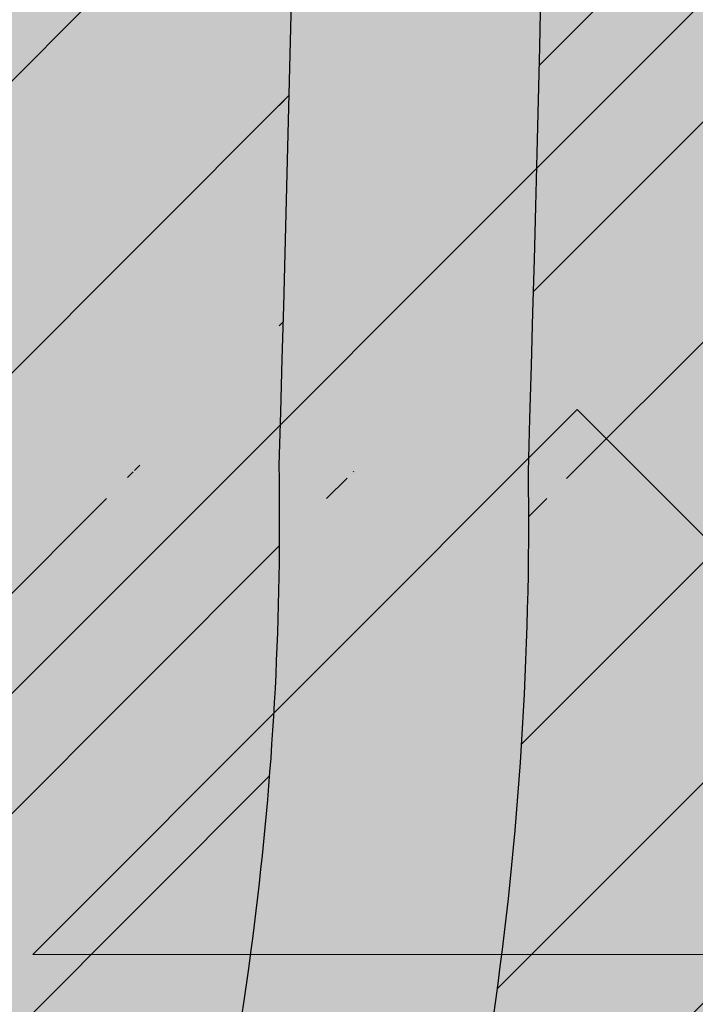
# Model space of a CAD drawing. Units: inches. Extents: x 844 to 2234, y 346 to 1084.
# Tile 11 of 93: x 1123.72 to 1124.585, y 691.183 to 692.442. Entities that reach past the tile are written whole.
import ezdxf

# ---------------------------------------------------------------- set-up
doc = ezdxf.new("R2010")
doc.units = ezdxf.units.IN
doc.header["$MEASUREMENT"] = 0
for name, color, linetype, lineweight in [('A-ANNO-DIMS', 2, 'Continuous', 18), ('furniture', 8, 'Continuous', 18), ('RA-AP-01$0$INT', 35, 'Continuous', 5)]:
    doc.layers.add(name, color=color, linetype=linetype, lineweight=lineweight)
doc.layers.add('RA-AP-01$0$FURN', color=3, linetype='Continuous')
doc.layers.add('RA-AP-01$0$WOOD', color=64, linetype='Continuous')
doc.styles.get("Standard").update_dxf_attribs({"font": 'arial.ttf'})
doc.dimstyles.get("Standard").update_dxf_attribs({"dimtxt": 6, "dimasz": 3, "dimexe": 0.18, "dimexo": 0.0625, "dimgap": 0.09, "dimtad": 0, "dimtih": 1, "dimtoh": 1, "dimdec": 1, "dimzin": 0, "dimdsep": 46, "dimlunit": 3, "dimtxsty": 'Standard', "dimblk": 'ARCHTICK', "dimcen": 0.09, "dimadec": 0, "dimazin": 0, "dimtfac": 1, "dimtdec": 1, "dimtofl": 0, "dimtmove": 0, "dimatfit": 3, "dimfxl": 1, "dimtolj": 1, "dimtzin": 0, "dimarcsym": 0})

# ---------------------------------------------------------------- blocks, each defined once
blk = doc.blocks.new('A$C18D01794')
at = {"layer": 'RA-AP-01$0$INT'}
h = blk.add_hatch(color=256, dxfattribs=at)
h.paths.add_polyline_path([(4.585917135068449, -6.356712009588271), (4.555206456959269, -6.35671200958746), (4.555206456959137, -6.387422687716308), (4.874495778835233, -6.706712009592356), (4.90520645695423, -6.676001331474049)])
h.paths.add_polyline_path([(5.255206456948813, -6.387422687716306), (5.255206456948682, -6.356712009605972), (5.224495778822613, -6.356712009605161), (4.905206456953498, -6.676001331474273), (4.935917135072151, -6.706712009592924)])
h.paths.add_polyline_path([(4.935917135072559, -6.706712009592068), (4.905206456953564, -6.737422687710376), (5.255206456951813, -7.087422687708613), (5.255206456951549, -7.026001331471008)])
h.paths.add_polyline_path([(4.555206456956399, -7.026001331471013), (4.555206456956134, -7.087422687708616), (4.905206456953821, -6.737422687710943), (4.874495778835166, -6.70671200959229)])
h = blk.add_hatch(color=256, dxfattribs=at)
h.paths.add_polyline_path([(4.585917135068448, -6.356712009588273), (4.614201406330596, -6.356712009589021), (4.668846067270487, -6.411356670531338), (4.723490728212344, -6.356712009591912), (4.771774999457151, -6.35671200959319), (4.826419660396886, -6.411356670535356), (4.862780050090322, -6.374996280843536), (4.844495778842715, -6.356712009595112), (4.862780050090411, -6.356712009595595), (4.905206456960182, -6.399138416468211), (4.947632863832445, -6.356712009597838), (4.965917135079675, -6.356712009598322), (4.947632863831759, -6.374996280845421), (4.983993253523576, -6.411356670538857), (5.038637914464627, -6.356712009600247), (5.08692218571208, -6.356712009601523), (5.141566846649976, -6.411356670541852), (5.196211507589851, -6.356712009604411), (5.224495778822615, -6.356712009605161), (4.905206456953975, -6.676001331473793)])
h.paths.add_polyline_path([(4.895206456956031, -6.637717060225675), (4.895206456958921, -6.528427738347902), (4.840561796018589, -6.583072399285802)], flags=16)
h.paths.add_polyline_path([(4.915206456955638, -6.637717060226121), (4.969851117895509, -6.583072399288678), (4.915206456957609, -6.528427738348344)], flags=16)
h.paths.add_polyline_path([(4.826419660395175, -6.568930263661755), (4.881064321335613, -6.514285602723745), (4.771774999456703, -6.514285602720857)], flags=16)
h.paths.add_polyline_path([(4.983993253519558, -6.568930263665262), (5.038637914460456, -6.514285602726792), (4.929348592581548, -6.514285602724816)], flags=16)
h.paths.add_polyline_path([(4.881064321336025, -6.494285602723742), (4.826419660397532, -6.439640941782821), (4.771774999457062, -6.494285602720859)], flags=16)
h.paths.add_polyline_path([(4.929348592582019, -6.494285602724817), (5.038637914460982, -6.494285602726792), (4.983993253522945, -6.439640941786327)], flags=16)
h.paths.add_polyline_path([(4.895206456960191, -6.480143467100443), (4.895206456962115, -6.407422687715913), (4.876922185715016, -6.389138416467584), (4.840561796021581, -6.425498806159401)], flags=16)
h.paths.add_polyline_path([(4.915206456958487, -6.480143467100889), (4.969851117899527, -6.425498806162279), (4.933490728206909, -6.389138416468043), (4.9152064569598, -6.40742268771434)], flags=16)
h.paths.add_polyline_path([(4.757632863832376, -6.480143467096812), (4.812277524772842, -6.425498806158772), (4.757632863834348, -6.370854145217844)], flags=16)
h.paths.add_polyline_path([(4.737632863832376, -6.480143467096286), (4.737632863834348, -6.370854145217375), (4.682988202893906, -6.425498806155385)], flags=16)
h.paths.add_polyline_path([(5.05278005008503, -6.480143467103376), (5.052780050087917, -6.370854145224413), (4.998135389146995, -6.425498806162908)], flags=16)
h.paths.add_polyline_path([(5.072780050085024, -6.480143467103744), (5.127424711025931, -6.42549880616527), (5.072780050087916, -6.370854145224832)], flags=16)
h.paths.add_polyline_path([(4.935917135072783, -6.706712009592292), (5.255206456948811, -6.387422687716309), (5.255206456948932, -6.415706958964177), (5.200561796010279, -6.470351619902839), (5.255206456949403, -6.524996280841948), (5.25520645694961, -6.5732805520894), (5.200561796009787, -6.627925213029239), (5.236922185702417, -6.664285602721864), (5.255206456949919, -6.646001331474357), (5.255206456949998, -6.664285602721898), (5.212780050078687, -6.706712009592262), (5.25520645695036, -6.749138416463932), (5.255206456950438, -6.767422687711313), (5.236922185702424, -6.749138416463297), (5.200561796009796, -6.785498806155928), (5.255206456950753, -6.840143467096874), (5.25520645695096, -6.888427738341682), (5.200561796010322, -6.943072399282328), (5.255206456951428, -6.997717060223427), (5.255206456951547, -7.026001331471006)])
h.paths.add_polyline_path([(5.042988202883395, -6.785498806155427), (5.097632863823085, -6.840143467095101), (5.097632863822622, -6.730854145216193)], flags=16)
h.paths.add_polyline_path([(5.028846067259663, -6.771356670531693), (5.083490728198774, -6.716712009592573), (4.974201406321001, -6.716712009593042)], flags=16)
h.paths.add_polyline_path([(5.117632863823087, -6.840143467095186), (5.172277524762331, -6.785498806155926), (5.11763286382262, -6.730854145216225)], flags=16)
h.paths.add_polyline_path([(5.08349072819877, -6.696712009593886), (5.028846067259652, -6.642067348654775), (4.974201406320998, -6.696712009593438)], flags=16)
h.paths.add_polyline_path([(5.131774999446817, -6.854285602718917), (5.186419660386065, -6.799640941779662), (5.241064321325782, -6.854285602719365)], flags=17)
h.paths.add_polyline_path([(5.131774999446228, -6.716712009592374), (5.186419660386065, -6.771356670532194), (5.222780050079488, -6.734996280838764), (5.204495778832781, -6.716712009592063)], flags=16)
h.paths.add_polyline_path([(5.097632863822613, -6.682569873970264), (5.097632863823061, -6.573280552091354), (5.042988202883383, -6.627925213031044)], flags=16)
h.paths.add_polyline_path([(5.131774999446899, -6.874285602718915), (5.241064321325809, -6.874285602719364), (5.186419660386591, -6.928930263658598)], flags=17)
h.paths.add_polyline_path([(5.131774999446226, -6.696712009594078), (5.204495778830767, -6.696712009594374), (5.22278005007868, -6.67842773834687), (5.186419660386049, -6.642067348654249)], flags=16)
h.paths.add_polyline_path([(5.11763286382262, -6.682569873970225), (5.17227752476232, -6.627925213030515), (5.117632863823064, -6.573280552091267)], flags=16)
h.paths.add_polyline_path([(5.186419660386069, -6.613783077405491), (5.241064321325754, -6.559138416465795), (5.131774999446791, -6.559138416466263)], flags=16)
h.paths.add_polyline_path([(5.131774999446872, -6.539138416466263), (5.24106432132578, -6.539138416465794), (5.186419660386554, -6.484493755526573)], flags=16)
h.paths.add_polyline_path([(5.255206456951811, -7.08742268770861), (5.255206456951895, -7.106712009588038), (4.555206456956052, -7.106712009588038), (4.555206456956136, -7.087422687708617), (4.905206456953973, -6.737422687710788)])
h.paths.add_polyline_path([(4.983993253513404, -6.8444937555241), (4.92934859257295, -6.899138416462108), (5.03863791445186, -6.899138416465014)], flags=16)
h.paths.add_polyline_path([(4.969851117889988, -6.83035161990006), (4.915206456952556, -6.775706958960171), (4.915206456949648, -6.884996280837944)], flags=16)
h.paths.add_polyline_path([(4.929348592572535, -6.919138416462105), (4.983993253511019, -6.973783077403037), (5.038637914451496, -6.919138416465012)], flags=16)
h.paths.add_polyline_path([(5.052780050074912, -6.93328055208906), (4.998135389134438, -6.987925213027088), (5.052780050072919, -7.042569873968025)], flags=16)
h.paths.add_polyline_path([(5.07278005007491, -6.933280552089588), (5.072780050072918, -7.042569873968497), (5.127424711013374, -6.987925213030498)], flags=16)
h.paths.add_polyline_path([(4.89520645695295, -6.775706958959721), (4.840561796013067, -6.830351619897157), (4.895206456950961, -6.884996280837494)], flags=16)
h.paths.add_polyline_path([(4.915206456948365, -6.933280552085403), (4.915206456946434, -7.006001331471951), (4.933490728192729, -7.024285602719066), (4.969851117886972, -6.987925213026453)], flags=16)
h.paths.add_polyline_path([(4.881064321327021, -6.899138416461022), (4.82641966038902, -6.84449375552057), (4.771774999448108, -6.899138416459029)], flags=16)
h.paths.add_polyline_path([(4.895206456950073, -6.933280552084951), (4.840561796009022, -6.987925213023558), (4.876922185700835, -7.024285602716997), (4.895206456948749, -7.006001331469487)], flags=16)
h.paths.add_polyline_path([(4.983993253510392, -7.0020673486505), (4.947632863816944, -7.038427738342319), (4.965917135064043, -7.05671200959023), (5.038637914448995, -7.056712009591555)], flags=16)
h.paths.add_polyline_path([(4.881064321326543, -6.91913841646102), (4.771774999447578, -6.919138416459031), (4.826419660385607, -6.973783077399508)], flags=16)
h.paths.add_polyline_path([(4.905206456946447, -7.014285602717636), (4.862780050074785, -7.056712009588352), (4.947632863816685, -7.056712009589775)], flags=16)
h.paths.add_polyline_path([(5.14156684663679, -7.002067348654549), (5.086922185696452, -7.056712009592438), (5.196211507574223, -7.056712009594425)], flags=16)
h.paths.add_polyline_path([(4.8264196603837, -7.002067348646972), (4.771774999442643, -7.056712009585575), (4.8444957788276, -7.056712009587508), (4.862780050075511, -7.038427738340416)], flags=16)
h.paths.add_polyline_path([(4.812277524760289, -6.98792521302292), (4.757632863822258, -6.933280552082447), (4.757632863819352, -7.042569873961408)], flags=16)
h.paths.add_polyline_path([(4.73763286382226, -6.933280552082079), (4.682988202881349, -6.987925213020536), (4.737632863819352, -7.04256987396099)], flags=16)
h.paths.add_polyline_path([(4.723490728195188, -7.056712009584289), (4.668846067257299, -7.002067348643949), (4.614201406317417, -7.056712009581383)], flags=16)
h.paths.add_polyline_path([(4.597632863829262, -6.706712009592262), (4.555206456957951, -6.664285602721896), (4.555206456958029, -6.646001331474357), (4.573490728205535, -6.664285602721864), (4.609851117898167, -6.627925213029238), (4.555206456958338, -6.573280552089402), (4.555206456958546, -6.524996280841952), (4.60985111789767, -6.470351619902839), (4.555206456959015, -6.415706958964177), (4.555206456959138, -6.387422687716309), (4.874495778835167, -6.70671200959229), (4.5552064569564, -7.026001331471015), (4.555206456956523, -6.997717060223433), (4.609851117897629, -6.94307239928233), (4.555206456956988, -6.888427738341681), (4.555206456957198, -6.840143467096881), (4.609851117898153, -6.78549880615593), (4.573490728205528, -6.749138416463297), (4.555206456957507, -6.76742268771132), (4.555206456957585, -6.749138416463933)])
h.paths.add_polyline_path([(4.712780050085332, -6.730854145216195), (4.712780050084863, -6.840143467095105), (4.767424711024555, -6.785498806155427)], flags=16)
h.paths.add_polyline_path([(4.726922185709173, -6.716712009592573), (4.781566846648288, -6.771356670531693), (4.836211507586949, -6.716712009593043)], flags=16)
h.paths.add_polyline_path([(4.692780050085327, -6.730854145216225), (4.638135389145619, -6.785498806155928), (4.692780050084865, -6.840143467095185)], flags=16)
h.paths.add_polyline_path([(4.726922185709182, -6.696712009593886), (4.836211507586949, -6.696712009593436), (4.7815668466483, -6.642067348654773)], flags=16)
h.paths.add_polyline_path([(4.678637914461726, -6.71671200959237), (4.605917135075169, -6.716712009592063), (4.587632863828464, -6.734996280838766), (4.623993253521887, -6.771356670532195)], flags=16)
h.paths.add_polyline_path([(4.712780050085336, -6.68256987397026), (4.767424711024568, -6.627925213031042), (4.71278005008489, -6.573280552091352)], flags=16)
h.paths.add_polyline_path([(4.678637914461726, -6.696712009594076), (4.623993253521899, -6.642067348654247), (4.587632863829271, -6.67842773834687), (4.605917135077185, -6.696712009594376)], flags=16)
h.paths.add_polyline_path([(4.692780050085336, -6.682569873970228), (4.692780050084889, -6.573280552091267), (4.638135389145632, -6.627925213030515)], flags=16)
h.paths.add_polyline_path([(4.623993253521885, -6.799640941779662), (4.678637914461131, -6.854285602718915), (4.56934859258217, -6.854285602719365)], flags=17)
h.paths.add_polyline_path([(4.623993253521901, -6.613783077405509), (4.678637914461158, -6.559138416466263), (4.569348592582195, -6.559138416465795)], flags=16)
h.paths.add_polyline_path([(4.678637914461051, -6.874285602718915), (4.623993253521361, -6.928930263658598), (4.569348592582143, -6.874285602719364)], flags=17)
h.paths.add_polyline_path([(4.678637914461076, -6.539138416466263), (4.623993253521399, -6.484493755526573), (4.569348592582167, -6.539138416465796)], flags=16)
h = blk.add_hatch(color=256, dxfattribs=at)
h.paths.add_polyline_path([(5.028846067259997, -6.642067348655121), (4.974201406321342, -6.696712009593783), (5.083490728199115, -6.69671200959423)])
h.paths.add_polyline_path([(4.974201406321344, -6.716712009593388), (5.028846067260004, -6.771356670532039), (5.083490728199117, -6.716712009592919)])
h.paths.add_polyline_path([(5.042988202883738, -6.785498806155768), (5.097632863823428, -6.840143467095449), (5.097632863822963, -6.73085414521654)])
h.paths.add_polyline_path([(5.117632863822961, -6.730854145216568), (5.117632863823428, -6.840143467095531), (5.172277524762674, -6.785498806156272)])
h.paths.add_polyline_path([(5.131774999446572, -6.716712009592718), (5.186419660386406, -6.77135667053254), (5.222780050079831, -6.734996280839116), (5.204495778833122, -6.716712009592409)])
h.paths.add_polyline_path([(5.236922185702764, -6.749138416463644), (5.200561796010139, -6.785498806156274), (5.255206456949971, -6.840143467096101), (5.255206456950271, -6.76742268771115)])
h.paths.add_polyline_path([(5.186419660386412, -6.799640941780006), (5.131774999447164, -6.854285602719262), (5.241064321326123, -6.854285602719711)])
h.paths.add_polyline_path([(5.131774999447238, -6.874285602719261), (5.186419660386934, -6.928930263658944), (5.241064321326153, -6.874285602719709)])
h.paths.add_polyline_path([(5.200561796010663, -6.943072399282675), (5.255206456949324, -6.997717060221329), (5.255206456949777, -6.888427738343558)])
h.paths.add_polyline_path([(5.21278005007903, -6.706712009592607), (5.255206456950223, -6.749138416463798), (5.255206456950696, -6.664285602721891)])
h.paths.add_polyline_path([(5.13177499944657, -6.696712009594424), (5.204495778831106, -6.696712009594723), (5.222780050079024, -6.678427738347219), (5.186419660386397, -6.642067348654592)])
h.paths.add_polyline_path([(5.117632863823405, -6.573280552091611), (5.117632863822955, -6.682569873970578), (5.172277524762665, -6.627925213030859)])
h.paths.add_polyline_path([(5.042988202883727, -6.627925213031387), (5.097632863822957, -6.682569873970603), (5.097632863823407, -6.573280552091697)])
h.paths.add_polyline_path([(5.131774999447135, -6.559138416466609), (5.186419660386394, -6.613783077405857), (5.241064321326097, -6.559138416466144)])
h.paths.add_polyline_path([(5.200561796010128, -6.627925213029584), (5.236922185702758, -6.664285602722211), (5.255206456950264, -6.646001331474705), (5.255206456949948, -6.573280552089752)])
h.paths.add_polyline_path([(5.186419660386895, -6.484493755526919), (5.131774999447213, -6.539138416466609), (5.241064321326127, -6.539138416466142)])
h.paths.add_polyline_path([(5.200561796010624, -6.470351619903183), (5.255206456949745, -6.524996280842298), (5.255206456949276, -6.415706958964523)])
for p, q in [((4.935917135072783, -6.706712009592292), (5.255206456951548, -7.026001331471007)), ((5.083490728198772, -6.716712009592574), (4.974201406321001, -6.716712009593042)), ((4.974201406321001, -6.716712009593042), (5.028846067259663, -6.771356670531693)), ((5.08349072819877, -6.716712009592578), (5.028846067259663, -6.771356670531693)), ((4.905206456953975, -6.737422687710788), (5.255206456951811, -7.087422687708611))]:
    blk.add_line(p, q, dxfattribs=at)
blk = doc.blocks.new('A$C32926AE1')
at = {"layer": 'RA-AP-01$0$FURN'}
h = blk.add_hatch(dxfattribs=at)
h.set_pattern_fill('ANSI31', color=256, scale=0.1, style=0)
h.set_pattern_definition([(45, (0, 0), (-0.0088388347648318, 0.0088388347648318), [])])
edge = h.paths.add_edge_path(flags=16)
edge.add_arc((4.904771284329206, 4.246793130718756), 0.2603971832811541, 75.22398030683196, 104.7760196931204)
edge.add_arc((4.904771284329206, 4.246793130718756), 0.2603971832811541, 75.223980306832, 104.77601969312039, ccw=False)
edge = h.paths.add_edge_path(flags=16)
edge.add_arc((4.904771284329206, 4.067062675376612), 0.2603971832811541, 255.2239803068796, 284.776019693168)
edge.add_arc((4.904771284329206, 4.067062675376612), 0.2603971832811541, 255.22398030687958, 284.77601969316805, ccw=False)
edge = h.paths.add_edge_path(flags=0)
edge.add_arc((4.904771284329206, 4.067062675376612), 0.2603971832811541, 255.2239803068796, 284.776019693168)
edge.add_arc((4.904771284329206, 4.067062675376612), 0.2603971832811541, 255.22398030687958, 284.77601969316805, ccw=False)
edge = h.paths.add_edge_path(flags=0)
edge.add_arc((4.904771284329206, 4.067062675376612), 0.2603971832811541, 255.2239803068796, 284.776019693168)
edge.add_arc((4.904771284329206, 4.067062675376612), 0.2603971832811541, 255.22398030687958, 284.77601969316805, ccw=False)
edge = h.paths.add_edge_path()
edge.add_arc((4.604388392048174, 4.588829985554312), 0.1599999999999918, 342.3781640246255, 354.4317409793762)
edge.add_arc((5.090145208887507, 4.43216705527679), 0.3503971832811637, 162.0091218307731, 180.3186872093483)
edge.add_arc((5.205154176610243, 4.588829985554953), 0.1599999999999917, 185.5682590208461, 197.6218359767349)
edge.add_arc((4.904771284329229, 4.246793130718735), 0.3503971832811761, 72.00912183053516, 107.9908781690354)
edge.add_arc((9.535952835716557, 4.28682295566602), 4.798342501046485, 178.2875002453811, 181.5576802719453)
edge.add_arc((4.719397359771122, 4.43216705527679), 0.3503971832811637, 359.6813127906516, 377.9908781692269)
edge.add_arc((9.535967292294904, 4.286822350292874), 4.778371420254705, 178.2965938931842, 181.5667745797229)
edge.add_arc((4.719397359771122, 4.43216705527679), 0.3303971832811637, 359.6813127906516, 377.9908781692269)
edge.add_arc((0.2735752763637294, 4.286822350292874), 4.7783714202547, 358.4332254202771, 361.7034061068158)
edge.add_arc((5.061434214606998, 4.732549947558029), 0.1600000000000254, 252.3781640250584, 264.4317409792362)
edge.add_arc((4.748108354051257, 4.732549947558012), 0.1600000000000541, 275.5682590208426, 287.6218359759532)
edge.add_arc((4.604388392048115, 4.588829985554317), 0.1800000000000505, 342.3567572500182, 349.3735009646207)
edge.add_arc((5.205154176610254, 4.588829985554976), 0.1800000000000069, 190.6264990356027, 197.6432427513933)
edge.add_arc((5.061434214607106, 4.732549947558013), 0.1800000000000424, 252.3567572496606, 259.3735009644582)
edge.add_arc((4.904771284329208, 4.246793130718737), 0.3303971832811676, 71.99844483668534, 108.0015551637021)
edge.add_arc((4.748108354051414, 4.732549947558045), 0.1800000000000547, 280.6264990355479, 287.6432427495938)
edge.add_arc((5.090145208887514, 4.432167055276789), 0.2803971832811691, 162.8706300666893, 180.816523289902)
edge.add_arc((4.719397359771136, 4.432167055276689), 0.2803971832811534, 359.183476710103, 377.1293699333214)
edge.add_arc((4.904771284329222, 4.246793130718737), 0.2803971832811769, 72.87063006672916, 107.1293699332334)
edge.add_arc((5.090145208887522, 4.432167055276788), 0.2603971832811776, 165.2239803068007, 180.9953123810312)
edge.add_arc((4.719397359771141, 4.432167055276699), 0.2603971832811458, 359.0046876189768, 374.7760196932087)
edge.add_arc((5.090145208887507, 4.43216705527679), 0.3303971832811637, 162.0091218307731, 180.3186872093483)
edge.add_arc((9.53595427642584, 4.285015535491528), 4.728345371032053, 178.265043920078, 181.5679956281801)
edge.add_arc((0.2735882922327999, 4.285015535491582), 4.728345371032045, 358.4320043718193, 361.7349560799204)
edge.add_arc((9.535953591267507, 4.284458026472751), 4.708343996644348, 178.2573054306777, 181.5704995759608)
edge.add_arc((0.273588977391114, 4.284458026472785), 4.708343996644358, 358.4295004240388, 361.7426945693213)
edge.add_arc((0.2735889773911131, 4.029397779622582), 4.708343996644359, 358.2573054306787, 361.5704995759613)
edge.add_arc((9.535953591267518, 4.029397779622618), 4.708343996644359, 178.4295004240391, 181.7426945693223)
edge.add_arc((0.2735882922327901, 4.028840270603786), 4.728345371032054, 358.2650439200796, 361.5679956281808)
edge.add_arc((9.53595427642584, 4.028840270603841), 4.728345371032054, 178.4320043718199, 181.7349560799219)
edge.add_arc((0.2735752763637302, 4.027033455802493), 4.778371420254699, 358.2965938931842, 361.5667745797229)
edge.add_arc((4.719397359771122, 3.881688750818578), 0.3303971832811637, 342.0091218307731, 360.3186872093484)
edge.add_arc((5.090145208887507, 3.881688750818578), 0.3303971832811637, 179.6813127906516, 197.9908781692269)
edge.add_arc((9.535967292294904, 4.027033455802493), 4.778371420254705, 178.433225420277, 181.7034061068158)
edge.add_arc((4.719397359771122, 3.881688750818578), 0.3503971832811637, 342.0091218307731, 360.3186872093484)
edge.add_arc((9.53595283571655, 4.027032850429349), 4.79834250104648, 178.4423197280546, 181.7124997546188)
edge.add_arc((4.719397359771141, 3.881688750818669), 0.2603971832811458, 345.2239803067913, 360.9953123810232)
edge.add_arc((5.090145208887522, 3.88168875081858), 0.2603971832811776, 179.0046876189687, 194.7760196931993)
edge.add_arc((4.904771284329222, 4.067062675376631), 0.2803971832811769, 252.8706300667665, 287.1293699332708)
edge.add_arc((4.719397359771136, 3.881688750818678), 0.2803971832811534, 342.8706300666787, 360.8165232898969)
edge.add_arc((5.090145208887514, 3.881688750818579), 0.2803971832811691, 179.183476710098, 197.1293699333106)
edge.add_arc((4.748108354051414, 3.581305858537323), 0.1800000000000547, 72.3567572504062, 79.37350096445199)
edge.add_arc((4.904771284329208, 4.067062675376631), 0.3303971832811676, 251.9984448362979, 288.0015551633146)
edge.add_arc((5.061434214607106, 3.581305858537355), 0.1800000000000424, 100.6264990355418, 107.6432427503394)
edge.add_arc((5.205154176610254, 3.725025820540392), 0.1800000000000069, 162.3567572486066, 169.3735009643972)
edge.add_arc((4.604388392048115, 3.725025820541051), 0.1800000000000505, 10.62649903537925, 17.64324274998182)
edge.add_arc((4.748108354051257, 3.581305858537356), 0.1600000000000541, 72.37816402404681, 84.43174097915735)
edge.add_arc((4.904771284329229, 4.067062675376632), 0.3503971832811761, 252.0091218309645, 287.9908781694648)
edge.add_arc((5.061434214606998, 3.581305858537339), 0.1600000000000254, 95.56825902076373, 107.6218359749416)
edge.add_arc((5.205154176610243, 3.725025820540414), 0.1599999999999917, 162.3781640232651, 174.4317409791539)
edge.add_arc((5.090145208887507, 3.881688750818578), 0.3503971832811637, 179.6813127906516, 197.9908781692269)
edge.add_arc((4.604388392048174, 3.725025820541056), 0.1599999999999918, 5.568259020623824, 17.62183597537444)
edge.add_arc((0.2735897329420762, 4.28682295566602), 4.798342501046482, 358.4423197280547, 361.7124997546188)
edge.add_arc((0.2735897329420691, 4.027032850429348), 4.798342501046489, 358.2875002453812, 361.5576802719453)
at = {"layer": 'RA-AP-01$0$WOOD'}
h = blk.add_hatch(color=256, dxfattribs=at)
h.dxf.hatch_style = 1
h.paths.add_polyline_path([(5.157430609644524, 4.573483066760929, -0.1009492694046607), (5.155401577623758, 4.593365984175333, -0.1842662638101597), (5.172249623284174, 4.638795604568598, 0.2056608120311276), (5.179560981299304, 4.661316324430096, 0.3614336704623542), (5.134352340494423, 4.706524965234944, 0.2056608120311297), (5.111831620632933, 4.699213607219793, -0.1842662638101113), (5.066402000239693, 4.682365561559342, -0.1055311479399994), (5.045656153913092, 4.68467289944697, 0.1567636581983829), (4.763886414745334, 4.684672899446966, -0.1055311479399895), (4.743140568418733, 4.68236556155934, -0.1842662638100833), (4.6977109480255, 4.69921360721979, 0.2056608120302612), (4.675190228164109, 4.706524965234949, 0.3614336704708441), (4.629981587358889, 4.66131632442871, 0.2056608120245944), (4.637292945374126, 4.638795604567974, -0.1842662638101024), (4.654140991034615, 4.59336598417475, -0.1009492694055169), (4.652111959013835, 4.573483066760181, 0.021410119221476), (4.629748025606143, 4.156712009541676, 0.0214101192214795), (4.652111959013809, 3.739940952323101, -0.1009492694059586), (4.654140991034615, 3.720058034908448, -0.1842662638100975), (4.637292945374126, 3.674628414515226, 0.2056608120245705), (4.629981587358889, 3.652107694654492, 0.3614336704708879), (4.675190228164113, 3.606899053848249, 0.2056608120302384), (4.697710948025501, 3.614210411863408, -0.1842662638100995), (4.743140568418738, 3.63105845752386, -0.1055311479402541), (4.763886414745388, 3.628751119636215, 0.1567636581983776), (5.045656153913137, 3.628751119636244, -0.1055311479397538), (5.066402000239692, 3.631058457523857, -0.1842662638101067), (5.111831620632931, 3.614210411863407, 0.2056608120310924), (5.134352340494417, 3.606899053848256, 0.3614336704624001), (5.179560981299307, 3.652107694653103, 0.2056608120311314), (5.172249623284175, 3.6746284145146, -0.1842662638101402), (5.155401577623758, 3.72005803490786, -0.1009492694051366), (5.15743060964455, 3.739940952322354, 0.0214101192215073), (5.179794543052287, 4.156712009541468, 0.0214101192215252)])
h.paths.add_polyline_path([(4.639748609479751, 4.156712009541513, 0.0213537860821624), (4.661970494867118, 3.741887061152232, -0.094075836301374), (4.664143710413708, 3.7196126951003, -0.1824818158568985), (4.644813765429836, 3.668037719127816, 0.2056608120245319), (4.639939526753007, 3.653023905887301, 0.3614336704710246), (4.676106439397173, 3.616856993242342, 0.2056608120302234), (4.691120252638095, 3.621731231919122, -0.1824818158602558), (4.742695228611606, 3.641061176902986, -0.1029891339458722), (4.766991894714349, 3.638256818950944, 0.156709409989566), (5.042550673941472, 3.638256818950105, -0.102989133958497), (5.066847340047078, 3.641061176902949, -0.1824818158594995), (5.118422316020358, 3.621731231919103, 0.2056608120311416), (5.133436129261316, 3.616856993242346, 0.3614336704621468), (5.169603041905217, 3.653023905886178, 0.2056608120310986), (5.164728803228477, 3.668037719127177, -0.1824818158565612), (5.145398858244737, 3.719612695099578, -0.0940758363009313), (5.147572073791232, 3.741887061151398, 0.0213537860822023), (5.169793959178681, 4.156712009541451, 0.0213537860822226), (5.147572073791203, 4.571536957931898, -0.0940758363005034), (5.145398858244737, 4.59381132398362, -0.1824818158565587), (5.164728803228476, 4.645386299956021, 0.2056608120311045), (5.169603041905216, 4.66040011319702, 0.3614336704621845), (5.133436129261313, 4.696567025840856, 0.2056608120310773), (5.118422316020359, 4.691692787164098, -0.182481815859508), (5.066847340047078, 4.67236284218025, -0.1029891339584606), (5.04255067394148, 4.675167200133092, 0.156709409989566), (4.766991894714357, 4.675167200132257, -0.1029891339458842), (4.742695228611611, 4.672362842180213, -0.1824818158602725), (4.691120252638095, 4.691692787164077, 0.2056608120302152), (4.676106439397174, 4.696567025840858, 0.3614336704710363), (4.639939526753005, 4.660400113195899, 0.2056608120245495), (4.644813765429837, 4.645386299955384, -0.1824818158568934), (4.664143710413708, 4.593811323982902, -0.0940758363009187), (4.661970494867149, 4.571536957931074, 0.021353786082177)], flags=16)
h.paths.add_polyline_path([(5.129794543052235, 4.432167055276933, -0.0141661062790638), (5.130152669293814, 4.156927903047693, -0.0141661062790647), (5.129794543052234, 3.881688750818433, -0.0785247771143638), (5.10979738006795, 3.755143611847103, 0.0945969212073497), (5.105408519571111, 3.717898134952927, 0.1043170707844957), (5.116074640131521, 3.670385395016088, 0.1043170707864965), (5.068561900193738, 3.681051515576561, 0.09459692119553), (5.031316423304057, 3.676662655080835, -0.1580239521427272), (4.778226145355827, 3.676662655080367, 0.0945969211986668), (4.740980668464973, 3.681051515576592, 0.1043170707882822), (4.693467928526415, 3.670385395015844, 0.1043170707867916), (4.704134049087309, 3.717898134953662, 0.0945969211972894), (4.69974518859162, 3.755143611844042, -0.0785247771163196), (4.679748025606343, 3.881688750818406, -0.0141661062790663), (4.679389899364763, 4.156927903047693, -0.0141661062790672), (4.679748025606343, 4.432167055276998, -0.0785247771163064), (4.699745188591625, 4.55871219425134, 0.094596921197333), (4.704134049087308, 4.595957671141738, 0.1043170707867205), (4.693467928526416, 4.643470411079523, 0.1043170707882628), (4.740980668464965, 4.632804290518776, 0.0945969211988114), (4.778226145355874, 4.637193151015016, -0.158023952142669), (5.031316423304015, 4.637193151014546, 0.0945969211956361), (5.068561900193736, 4.632804290518806, 0.1043170707864979), (5.11607464013152, 4.643470411079278, 0.1043170707844617), (5.105408519571112, 4.595957671142455, 0.0945969212074597), (5.109797380067959, 4.558712194248236, -0.0785247771143467)], flags=0)
h.paths.add_polyline_path([(5.119794532311105, 4.432259799204851, -0.0142000800617244), (5.120156169157484, 4.156927903047701, -0.0142000800617277), (5.119794532311105, 3.881596006890482, -0.0784894509520253), (5.100273383573699, 3.758192358677797, 0.0940138827242913), (5.095413455884425, 3.717477693979438, 0.0606271852308753), (5.099615656341024, 3.686844378806616, 0.0606271852322524), (5.068982341167493, 3.691046579263239, 0.0940138827010453), (5.028267676478798, 3.686186651576848, -0.1580706864508061), (4.781274892180912, 3.686186651576435, 0.0940138827026903), (4.740560227491556, 3.691046579263279, 0.0606271852339895), (4.709926912317155, 3.686844378806508, 0.0606271852329405), (4.714129112773991, 3.717477693980356, 0.094013882701304), (4.709269185087677, 3.758192358669163, -0.0784894509577193), (4.689748036347473, 3.881596006890469, -0.014200080061729), (4.689386399501094, 4.156927903047709, -0.0142000800617217), (4.689748036347473, 4.432259799204808, -0.078489450957724), (4.709269185087651, 4.555663447426125, 0.0940138827014585), (4.714129112773992, 4.596378112114996, 0.0606271852329731), (4.709926912317154, 4.62701142728886, 0.0606271852340196), (4.74056022749157, 4.622809226832087, 0.0940138827024997), (4.781274892180847, 4.627669154518912, -0.1580706864508359), (5.028267676478777, 4.627669154518526, 0.0940138827010946), (5.068982341167492, 4.622809226832129, 0.060627185232254), (5.099615656341024, 4.627011427288751, 0.0606271852308727), (5.095413455884425, 4.59637811211593, 0.0940138827241088), (5.100273383573675, 4.555663447417647, -0.0784894509520978)], flags=0)
h.paths.add_polyline_path([(5.06978912287499, 4.430218106756144, -0.014241683694547), (5.070173729147532, 4.156927903047672, -0.0142416836945458), (5.06978912287499, 3.883637699339223, -0.0800609523125196), (5.052662118612511, 3.773463122773442, 0.0526421978001116), (5.04590916754064, 3.740550867606997, 0.0526421977992423), (5.012996912374707, 3.73379791653534, -0.1583028414718258), (4.796545656286308, 3.73379791653451, 0.0526421978034211), (4.763633401117837, 3.740550867607021, 0.0526421978018622), (4.756880450045755, 3.773463122774558, -0.0800609523117106), (4.739753445783639, 3.883637699339268, -0.0142416836945435), (4.739368839511098, 4.156927903047671, -0.0142416836945477), (4.739753445783639, 4.430218106756155, -0.0800609523116345), (4.75688045004574, 4.540392683320762, 0.052642197801941), (4.763633401117837, 4.573304938488346, 0.0526421978035071), (4.796545656286361, 4.580057889560873, -0.1583028414717561), (5.012996912374669, 4.580057889560039, 0.0526421977993048), (5.04590916754064, 4.57330493848837, 0.0526421978002057), (5.052662118612529, 4.540392683321868, -0.080060952312477)], flags=0)
h.paths.add_polyline_path([(5.049789715110557, 4.43038092723357, -0.0143097550741839), (5.05018085590259, 4.156927903047715, -0.0143097550741854), (5.049789715110558, 3.883474878861827, -0.0800685599149176), (5.03362098255317, 3.779581877367999, 0.0306258898956367), (5.028241146483733, 3.758218888663947, 0.0306258898977031), (5.006878157778253, 3.75283905259408, -0.1583983521624096), (4.802664410878162, 3.752839052594731, 0.0306258898946014), (4.781301422174808, 3.758218888663924, 0.0306258898967912), (4.775921586105202, 3.779581877368794, -0.080068559914251), (4.759752853548071, 3.883474878861786, -0.0143097550741854), (4.759361712756037, 4.156927903047671, -0.0143097550741854), (4.759752853548071, 4.430380927233557, -0.0800685599142479), (4.775921586105193, 4.534273928726546, 0.0306258898968306), (4.781301422174808, 4.555636917431444, 0.0306258898945754), (4.802664410878143, 4.561016753500631, -0.1583983521624168), (5.006878157778244, 4.561016753501291, 0.0306258898977177), (5.028241146483733, 4.555636917431421, 0.0306258898958182), (5.03362098255321, 4.534273928727244, -0.080068559914796)], flags=0)
h.paths.add_polyline_path([(4.999766070382627, 4.428171244713864, -0.0143443147609634), (5.000198441819402, 4.156927903047689, -0.0143443147609612), (4.999766070382627, 3.885684561381556, -0.0784641635803329), (4.987356730658798, 3.799103304488872, -0.1506053783831347), (4.822185837999821, 3.79910330448882, -0.0784641635803318), (4.809776498276007, 3.885684561381509, -0.014344314760963), (4.809344126839227, 4.156927903047677, -0.0143443147609645), (4.809776498276007, 4.428171244713873, -0.0784641635803192), (4.822185837999822, 4.514752501606549, -0.1506053783831338), (4.987356730658798, 4.514752501606494, -0.078464163580285)], flags=0)
h.paths.add_polyline_path([(4.979755254238824, 4.42764379880488, -0.0143772539198268), (4.980205517789977, 4.156927903047693, -0.0143772539198275), (4.979755254238824, 3.886212007290489, -0.0689242507424422), (4.971183264704897, 3.815276770442801, -0.1296645318904179), (4.838359303953726, 3.815276770442746, -0.0689242507424186), (4.829787314419809, 3.886212007290419, -0.0143772539198292), (4.829337050868653, 4.156927903047653, -0.0143772539198325), (4.829787314419809, 4.427643798804946, -0.0689242507424211), (4.838359303953725, 4.498579035652621, -0.1296645318904187), (4.971183264704897, 4.498579035652565, -0.0689242507424401)], flags=0)
h = blk.add_hatch(color=256, dxfattribs=at)
h.dxf.hatch_style = 1
h.paths.add_polyline_path([(5.145398858244737, 4.59381132398362, -0.1824818158565616), (5.164728803228476, 4.645386299956021, 0.2056608120311045), (5.169603041905216, 4.66040011319702, 0.3614336704621845), (5.133436129261313, 4.696567025840856, 0.2056608120310773), (5.118422316020359, 4.691692787164098, -0.182481815859508), (5.066847340047078, 4.67236284218025, -0.1029891339584606), (5.04255067394148, 4.675167200133092, 0.156709409989566), (4.766991894714357, 4.675167200132257, -0.1029891339458842), (4.742695228611611, 4.672362842180213, -0.1824818158602725), (4.691120252638095, 4.691692787164077, 0.2056608120302152), (4.676106439397174, 4.696567025840858, 0.3614336704710363), (4.639939526753005, 4.660400113195899, 0.2056608120245495), (4.644813765429837, 4.645386299955384, -0.1824818158568934), (4.664143710413708, 4.593811323982902, -0.0940758363009187), (4.661970494867149, 4.571536957931074, 0.0213537860821772), (4.639748609479751, 4.156712009541507, 0.0213537860821625), (4.661970494867119, 3.741887061152226, -0.0940758363013071), (4.664143710413708, 3.719612695100309, -0.1824818158569294), (4.644813765429836, 3.668037719127816, 0.2056608120245319), (4.639939526753007, 3.653023905887301, 0.3614336704710246), (4.676106439397173, 3.616856993242342, 0.2056608120302234), (4.691120252638095, 3.621731231919122, -0.1824818158602558), (4.742695228611606, 3.641061176902986, -0.1029891339458722), (4.766991894714349, 3.638256818950944, 0.156709409989566), (5.042550673941472, 3.638256818950105, -0.102989133958497), (5.066847340047078, 3.641061176902949, -0.1824818158594995), (5.118422316020358, 3.621731231919103, 0.2056608120311416), (5.133436129261316, 3.616856993242346, 0.3614336704621468), (5.169603041905217, 3.653023905886178, 0.2056608120310986), (5.164728803228477, 3.668037719127177, -0.1824818158565612), (5.145398858244737, 3.719612695099578, -0.0940758363009313), (5.147572073791232, 3.741887061151398, 0.0213537860822023), (5.169793959178681, 4.156712009541451, 0.0213537860822226), (5.147572073791203, 4.571536957931898, -0.0940758363004996)])
h.paths.add_polyline_path([(5.109797380067958, 4.55871219424824, -0.0785247771143472), (5.129794543052234, 4.432167055276936, -0.0141661062790644), (5.130152669293814, 4.156927903047685, -0.014166106279066), (5.129794543052234, 3.881688750818401, -0.0785247771143517), (5.109797380067946, 3.755143611847092, 0.0945969212073132), (5.105408519571111, 3.717898134952929, 0.1043170707844995), (5.116074640131521, 3.670385395016088, 0.1043170707864965), (5.068561900193738, 3.681051515576561, 0.09459692119553), (5.031316423304057, 3.676662655080835, -0.1580239521427272), (4.778226145355827, 3.676662655080367, 0.0945969211986668), (4.740980668464973, 3.681051515576592, 0.1043170707882822), (4.693467928526415, 3.670385395015844, 0.1043170707867916), (4.704134049087309, 3.717898134953662, 0.0945969211972894), (4.69974518859162, 3.755143611844042, -0.0785247771163196), (4.679748025606343, 3.881688750818406, -0.0141661062790663), (4.679389899364763, 4.156927903047693, -0.0141661062790672), (4.679748025606343, 4.432167055276998, -0.0785247771163064), (4.699745188591625, 4.55871219425134, 0.094596921197333), (4.704134049087308, 4.595957671141738, 0.1043170707867205), (4.693467928526416, 4.643470411079523, 0.1043170707882628), (4.740980668464965, 4.632804290518776, 0.0945969211988114), (4.778226145355874, 4.637193151015016, -0.158023952142669), (5.031316423304015, 4.637193151014546, 0.0945969211956361), (5.068561900193736, 4.632804290518806, 0.1043170707864979), (5.11607464013152, 4.643470411079278, 0.1043170707844617), (5.105408519571112, 4.595957671142455, 0.0945969212074504)], flags=16)
h.paths.add_polyline_path([(5.100273383573655, 4.55566344741771, -0.0784894509521388), (5.119794532311105, 4.432259799204852, -0.0142000800617252), (5.120156169157484, 4.156927903047686, -0.014200080061726), (5.119794532311105, 3.881596006890502, -0.0784894509520446), (5.100273383573696, 3.758192358677786, 0.0940138827242721), (5.095413455884425, 3.717477693979436, 0.0606271852308692), (5.099615656341024, 3.686844378806616, 0.0606271852322522), (5.068982341167493, 3.691046579263239, 0.0940138827010453), (5.028267676478798, 3.686186651576848, -0.1580706864508061), (4.781274892180912, 3.686186651576435, 0.0940138827026903), (4.740560227491556, 3.691046579263279, 0.0606271852339895), (4.709926912317155, 3.686844378806508, 0.0606271852329405), (4.714129112773991, 3.717477693980356, 0.094013882701304), (4.709269185087677, 3.758192358669163, -0.0784894509577193), (4.689748036347473, 3.881596006890469, -0.014200080061729), (4.689386399501094, 4.156927903047709, -0.0142000800617217), (4.689748036347473, 4.432259799204808, -0.078489450957724), (4.709269185087651, 4.555663447426125, 0.0940138827014585), (4.714129112773992, 4.596378112114996, 0.0606271852329731), (4.709926912317154, 4.62701142728886, 0.0606271852340196), (4.74056022749157, 4.622809226832087, 0.0940138827024997), (4.781274892180847, 4.627669154518912, -0.1580706864508359), (5.028267676478777, 4.627669154518526, 0.0940138827010946), (5.068982341167492, 4.622809226832129, 0.060627185232254), (5.099615656341024, 4.627011427288751, 0.0606271852308727), (5.095413455884425, 4.59637811211593, 0.094013882723957)], flags=0)
h.paths.add_polyline_path([(5.04590916754064, 4.57330493848837, 0.0526421978002057), (5.052662118612529, 4.540392683321868, -0.0800609523124783), (5.06978912287499, 4.430218106756142, -0.0142416836945469), (5.070173729147532, 4.156927903047672, -0.0142416836945458), (5.06978912287499, 3.883637699339223, -0.0800609523125196), (5.052662118612511, 3.773463122773442, 0.0526421978001116), (5.04590916754064, 3.740550867606997, 0.0526421977992423), (5.012996912374707, 3.73379791653534, -0.1583028414718258), (4.796545656286308, 3.73379791653451, 0.0526421978034211), (4.763633401117837, 3.740550867607021, 0.0526421978018622), (4.756880450045755, 3.773463122774558, -0.0800609523117106), (4.739753445783639, 3.883637699339268, -0.0142416836945435), (4.739368839511098, 4.156927903047671, -0.0142416836945477), (4.739753445783639, 4.430218106756155, -0.0800609523116345), (4.75688045004574, 4.540392683320762, 0.052642197801941), (4.763633401117837, 4.573304938488346, 0.0526421978035071), (4.796545656286361, 4.580057889560873, -0.1583028414717561), (5.012996912374669, 4.580057889560039, 0.0526421977993048)], flags=0)
h.paths.add_polyline_path([(5.028241146483733, 4.555636917431422, 0.0306258898956949), (5.033620982553182, 4.534273928727329, -0.0800685599148649), (5.049789715110557, 4.430380927233569, -0.0143097550741839), (5.05018085590259, 4.156927903047715, -0.0143097550741854), (5.049789715110558, 3.883474878861827, -0.0800685599149176), (5.03362098255317, 3.779581877367999, 0.0306258898956367), (5.028241146483733, 3.758218888663947, 0.0306258898977031), (5.006878157778253, 3.75283905259408, -0.1583983521624096), (4.802664410878162, 3.752839052594731, 0.0306258898946014), (4.781301422174808, 3.758218888663924, 0.0306258898967912), (4.775921586105202, 3.779581877368794, -0.080068559914251), (4.759752853548071, 3.883474878861786, -0.0143097550741854), (4.759361712756037, 4.156927903047671, -0.0143097550741854), (4.759752853548071, 4.430380927233557, -0.0800685599142479), (4.775921586105193, 4.534273928726546, 0.0306258898968306), (4.781301422174808, 4.555636917431444, 0.0306258898945754), (4.802664410878143, 4.561016753500631, -0.1583983521624168), (5.006878157778244, 4.561016753501291, 0.0306258898977174)], flags=0)
h.paths.add_polyline_path([(4.987356730658798, 4.514752501606494, -0.0784641635803018), (4.999766070382627, 4.428171244713845, -0.0143443147609637), (5.000198441819402, 4.156927903047665, -0.0143443147609622), (4.999766070382628, 3.885684561381514, -0.0784641635802952), (4.987356730658797, 3.799103304488872, -0.1506053783831338), (4.822185837999821, 3.799103304488819, -0.0784641635803342), (4.809776498276007, 3.885684561381512, -0.0143443147609628), (4.809344126839227, 4.156927903047676, -0.0143443147609646), (4.809776498276007, 4.428171244713873, -0.0784641635803192), (4.822185837999822, 4.514752501606549, -0.1506053783831338)], flags=0)
h.paths.add_polyline_path([(4.971183264704897, 4.498579035652566, -0.0689242507424384), (4.979755254238824, 4.427643798804883, -0.0143772539198276), (4.980205517789977, 4.15692790304768, -0.0143772539198258), (4.979755254238823, 3.88621200729051, -0.0689242507424628), (4.971183264704897, 3.815276770442801, -0.129664531890417), (4.838359303953726, 3.815276770442746, -0.0689242507424186), (4.829787314419809, 3.886212007290419, -0.0143772539198292), (4.829337050868653, 4.156927903047653, -0.0143772539198325), (4.829787314419809, 4.427643798804946, -0.0689242507424211), (4.838359303953725, 4.498579035652621, -0.1296645318904187)], flags=0)
h = blk.add_hatch(dxfattribs=at)
h.set_pattern_fill('ANSI31', color=256, scale=0.05, style=0)
h.set_pattern_definition([(45, (0, 0), (-0.0044194173824159, 0.0044194173824159), [])])
h.paths.add_polyline_path([(5.130152669293814, 4.156927903047704, 0.0141661062790657), (5.129794543052234, 4.432167055276982, 0.0777827904001433), (5.110168979996553, 4.557559993161921, -0.0976515123401879), (5.105408519571111, 4.595957671142454, -0.1043170707844687), (5.116074640131522, 4.64347041107928), (5.099615656341024, 4.627011427288751, 0.0606271852308727), (5.095413455884425, 4.59637811211593, 0.0940138827241088), (5.100273383573675, 4.555663447417647, -0.0784894509520972), (5.119794532311105, 4.432259799204852, -0.0142000800617252), (5.120156169157484, 4.156927903047686, -0.014200080061726), (5.119794532311105, 3.881596006890502, -0.0784894509520446), (5.100273383573696, 3.758192358677786, 0.0940138827242721), (5.095413455884425, 3.717477693979436, 0.0606271852308692), (5.099615656341024, 3.686844378806616), (5.116074640131519, 3.67038539501609, -0.1043170707844594), (5.105408519571112, 3.717898134952912, -0.0976515123401594), (5.11016897999655, 3.756295812933435, 0.0777827904001654), (5.129794543052234, 3.881688750818409, 0.0141661062790665)])
h.paths.add_polyline_path([(5.030164222210597, 3.676291055149937, -0.0976515123472002), (5.068561900193739, 3.681051515576561, -0.1043170707864927), (5.116074640131521, 3.670385395016088), (5.099615656341024, 3.686844378806616, 0.0606271852322522), (5.068982341167493, 3.691046579263239, 0.0940138827010453), (5.028267676478798, 3.686186651576848, -0.1580706864508061), (4.781274892180912, 3.686186651576435, 0.0940138827026903), (4.740560227491556, 3.691046579263279, 0.0606271852339913), (4.709926912317154, 3.686844378806508), (4.693467928526416, 3.670385395015845, -0.1043170707882796), (4.740980668464973, 3.681051515576592, -0.0976515123427246), (4.779378346446416, 3.676291055150394, 0.156512506893803)])
h.paths.add_polyline_path([(4.689748036347473, 3.881596006890472, -0.014200080061729), (4.689386399501094, 4.156927903047712, -0.0142000800617195), (4.689748036347473, 4.432259799204768, -0.078489450957742), (4.709269185087648, 4.555663447426114, 0.0940138827014821), (4.714129112773992, 4.596378112114995, 0.0606271852329748), (4.709926912317154, 4.62701142728886), (4.693467928526414, 4.643470411079524, -0.1043170707867939), (4.704134049087309, 4.595957671141706, -0.09765151234893), (4.699373588660725, 4.557559993157876, 0.0777827903975372), (4.679748025606343, 4.432167055276987, 0.0141661062790675), (4.679389899364763, 4.156927903047675, 0.0141661062790641), (4.679748025606343, 3.88168875081843, 0.0777827903975637), (4.699373588660724, 3.756295812937497, -0.0976515123490278), (4.704134049087308, 3.717898134953629, -0.1043170707867196), (4.693467928526416, 3.670385395015845), (4.709926912317155, 3.686844378806508, 0.0606271852329413), (4.714129112773991, 3.717477693980357, 0.0940138827013084), (4.709269185087676, 3.758192358669166, -0.0784894509577192)])
h.paths.add_polyline_path([(4.779378346446434, 4.63756475094498, -0.0976515123427943), (4.740980668464964, 4.632804290518776, -0.1043170707882609), (4.693467928526416, 4.643470411079523), (4.709926912317154, 4.62701142728886, 0.0606271852340196), (4.74056022749157, 4.622809226832087, 0.0940138827024997), (4.781274892180847, 4.627669154518912, -0.1580706864508359), (5.028267676478777, 4.627669154518526, 0.0940138827010946), (5.068982341167492, 4.622809226832129, 0.060627185232254), (5.099615656341024, 4.627011427288751), (5.116074640131521, 4.643470411079279, -0.1043170707865022), (5.068561900193735, 4.632804290518806, -0.0976515123475899), (5.030164222210446, 4.637564750945479, 0.1565125068936924)])
h = blk.add_hatch(dxfattribs=at)
h.set_pattern_fill('ANSI32', color=256, scale=0.2, style=0)
h.set_pattern_definition([(45, (0, 0), (-0.0530330085889911, 0.0530330085889911), []), (45, (0.035355339, 0), (-0.0530330085889911, 0.0530330085889911), [])])
h.paths.add_polyline_path([(5.119794532311105, 4.432259799204823, 0.0777015974868765), (5.10065834347252, 4.554469821747928, -0.0968902511992216), (5.095413455884425, 4.596378112115931, -0.060627185230871), (5.099615656341024, 4.627011427288751, -0.060627185232254), (5.068982341167492, 4.622809226832129, -0.0968902512198245), (5.027074050790956, 4.628054114423209, 0.1564657949319105), (4.782468517866163, 4.628054114422785, -0.0968902512152247), (4.740560227491555, 4.622809226832088, -0.0606271852339878), (4.709926912317155, 4.627011427288859, -0.0606271852329413), (4.714129112773991, 4.596378112115011, -0.0968902512205338), (4.708884225182929, 4.554469821738175, 0.0777015974804443), (4.689748036347473, 4.43225979920482, 0.0142000800617215), (4.689386399501094, 4.156927903047726, 0.0142000800617273), (4.689748036347473, 3.88159600689052, 0.077701597480541), (4.708884225182985, 3.759385984357019, -0.096890251220082), (4.714129112773992, 3.717477693980371, -0.0606271852329731), (4.709926912317154, 3.686844378806507, -0.060627185233988), (4.740560227491554, 3.691046579263279, -0.0968902512152569), (4.782468517866175, 3.685801691672578, 0.1564657949319236), (5.027074050790988, 3.685801691672169, -0.0968902512197451), (5.068982341167491, 3.691046579263239, -0.0606271852322557), (5.099615656341024, 3.686844378806616, -0.0606271852308727), (5.095413455884425, 3.717477693979438, -0.0968902511991229), (5.100658343472507, 3.7593859843474, 0.0777015974868745), (5.119794532311105, 3.8815960068905, 0.014200080061726), (5.120156169157484, 4.156927903047685, 0.0142000800617238)])
h.paths.add_polyline_path([(5.070173729147531, 4.156927903047684, -0.0142416836945481), (5.06978912287499, 3.883637699339191, -0.0800609523125107), (5.052662118612505, 3.773463122773424, 0.0526421978000811), (5.04590916754064, 3.740550867606997, 0.0526421977993214), (5.012996912374658, 3.733797916535325, -0.1583028414717916), (4.796545656286304, 3.733797916534512, 0.0526421978034138), (4.763633401117837, 3.740550867607021, 0.0526421978018622), (4.756880450045755, 3.773463122774558, -0.0800609523117106), (4.739753445783639, 3.883637699339268, -0.0142416836945435), (4.739368839511098, 4.156927903047671, -0.0142416836945477), (4.739753445783639, 4.430218106756155, -0.0800609523116345), (4.75688045004574, 4.540392683320762, 0.052642197801941), (4.763633401117837, 4.573304938488346, 0.0526421978035071), (4.796545656286361, 4.580057889560873, -0.1583028414717561), (5.012996912374669, 4.580057889560039, 0.0526421977993048), (5.04590916754064, 4.57330493848837, 0.0526421978002057), (5.052662118612529, 4.540392683321868, -0.0800609523124783), (5.06978912287499, 4.430218106756142, -0.0142416836945463)], flags=16)
h.paths.add_polyline_path([(5.050180855902591, 4.156927903047686, -0.0143097550741856), (5.049789715110558, 3.883474878861795, -0.0800685599148126), (5.033620982553202, 3.7795818773681, 0.0306258898957837), (5.028241146483733, 3.758218888663947, 0.0306258898977031), (5.006878157778253, 3.75283905259408, -0.1583983521624096), (4.802664410878162, 3.752839052594731, 0.0306258898946014), (4.781301422174808, 3.758218888663924, 0.0306258898967912), (4.775921586105202, 3.779581877368794, -0.080068559914251), (4.759752853548071, 3.883474878861786, -0.0143097550741854), (4.759361712756037, 4.156927903047671, -0.0143097550741854), (4.759752853548071, 4.430380927233557, -0.0800685599142479), (4.775921586105193, 4.534273928726546, 0.0306258898968306), (4.781301422174808, 4.555636917431444, 0.0306258898945754), (4.802664410878143, 4.561016753500631, -0.1583983521624168), (5.006878157778244, 4.561016753501291, 0.0306258898977177), (5.028241146483733, 4.555636917431421, 0.0306258898958182), (5.03362098255321, 4.534273928727244, -0.0800685599147973), (5.049789715110557, 4.430380927233568, -0.0143097550741854)], flags=0)
h.paths.add_polyline_path([(5.000198441819402, 4.15692790304769, -0.0143443147609622), (4.999766070382627, 3.885684561381539, -0.0784641635803169), (4.987356730658798, 3.799103304488873, -0.1506053783831347), (4.822185837999821, 3.79910330448882, -0.0784641635803318), (4.809776498276007, 3.885684561381509, -0.014344314760963), (4.809344126839227, 4.156927903047677, -0.0143443147609645), (4.809776498276007, 4.428171244713873, -0.0784641635803192), (4.822185837999822, 4.514752501606549, -0.1506053783831338), (4.987356730658798, 4.514752501606494, -0.0784641635803018), (4.999766070382627, 4.428171244713845, -0.0143443147609624)], flags=0)
h.paths.add_polyline_path([(4.980205517789976, 4.156927903047707, -0.0143772539198295), (4.979755254238824, 3.886212007290466, -0.06892425074242), (4.971183264704897, 3.815276770442801, -0.129664531890417), (4.838359303953726, 3.815276770442746, -0.0689242507424186), (4.829787314419809, 3.886212007290419, -0.0143772539198292), (4.829337050868653, 4.156927903047653, -0.0143772539198325), (4.829787314419809, 4.427643798804946, -0.0689242507424211), (4.838359303953725, 4.498579035652621, -0.1296645318904187), (4.971183264704897, 4.498579035652565, -0.0689242507424418), (4.979755254238824, 4.427643798804878, -0.0143772539198259)], flags=0)
for centre, radius, start, end in [((0.2735889773911131, 4.029397779622582), 4.708343996644359, 358.2573054306787, 1.570499575961277), ((0.2735882922327901, 4.028840270603786), 4.728345371032054, 358.2650439200796, 1.567995628180738), ((4.719397359771141, 3.881688750818669), 0.2603971832811458, 345.2239803067913, 0.9953123810231653), ((4.719397359771136, 3.881688750818678), 0.2803971832811534, 342.8706300666787, 0.8165232898969792)]:
    blk.add_arc(centre, radius, start, end, dxfattribs=at)
blk = doc.blocks.new('A$C5D2F253E')
at = {"layer": 'RA-AP-01$0$FURN', "xscale": -0.7999999999883585, "yscale": 0.7999999999883585, "zscale": 0.8, "rotation": 90}
blk.add_blockref('A$C18D01794', (-5.687757199772477, 4.75791982714071), dxfattribs=at)
at = {"layer": 'RA-AP-01$0$WOOD', "rotation": 270}
blk.add_blockref('A$C32926AE1', (-4.161339601644158, 5.73852594588169), dxfattribs=at)
blk = doc.blocks.new('_ArchTick')
at = {"color": 0, "linetype": 'ByBlock', "const_width": 0.15}
blk.add_lwpolyline([(-0.5, -0.5), (0.5, 0.5)], dxfattribs=at)
blk = doc.blocks.new('*D144')
at = {"layer": 'A-ANNO-DIMS', "color": 0, "lineweight": -2, "transparency": 16777216}
for p, q in [((1096.615948, 439.3732739999999), (1096.615948, 1074.743301)), ((1143.115948, 492.373274), (1143.115948, 1074.743301)), ((1096.615948, 1074.563301), (1102.481950728513, 1074.563301)), ((1143.115948, 1074.563301), (1137.249945271487, 1074.563301))]:
    blk.add_line(p, q, dxfattribs=at)
at = {"layer": 'Defpoints', "color": 0, "transparency": 16777216}
for p in [(1143.115948, 1074.563301), (1143.115948, 492.3107739999999), (1096.615948, 439.3107739999999)]:
    blk.add_point(p, dxfattribs=at)
at = {"layer": 'A-ANNO-DIMS', "color": 0, "lineweight": -2, "transparency": 16777216, "xscale": 3, "yscale": 3, "zscale": 3, "rotation": 180}
blk.add_blockref('_ArchTick', (1096.615948, 1074.563301), dxfattribs=at)
at = {"layer": 'A-ANNO-DIMS', "color": 0, "lineweight": -2, "transparency": 16777216, "xscale": 3, "yscale": 3, "zscale": 3}
blk.add_blockref('_ArchTick', (1143.115948, 1074.563301), dxfattribs=at)
at = {"layer": 'A-ANNO-DIMS', "color": 0, "transparency": 16777216, "insert": (1119.865948, 1074.563301), "char_height": 6, "attachment_point": 5}
blk.add_mtext('\\A1;3\'-10 1/2"', dxfattribs=at)

msp = doc.modelspace()

# ---------------------------------------------------------------- block references
at = {"layer": 'furniture', "xscale": 15.94108302203742, "yscale": 15.94108302203742, "zscale": 15.94108302203742, "rotation": 90}
msp.add_blockref('A$C5D2F253E', (1136.147844094663, 696.2584716700112), dxfattribs=at)

# ---------------------------------------------------------------- dimensions: what is measured, and where the dimension line sits
at = {"layer": 'A-ANNO-DIMS'}
dim = msp.add_linear_dim(base=(1143.115948, 1074.563301), p1=(1096.615948, 439.3107739999999), p2=(1143.115948, 492.3107739999999), dimstyle='Standard', override={"dimdec": 1, "dimlfac": 1, "dimrnd": 0, "dimzin": 1, "dimdsep": 46, "dimlunit": 4, "dimfrac": 2}, dxfattribs=at)
dim.commit()
dim.dimension.update_dxf_attribs({"geometry": '*D144', "text_midpoint": (1119.865948, 1074.563301)})

doc.saveas('drawing.dxf')
